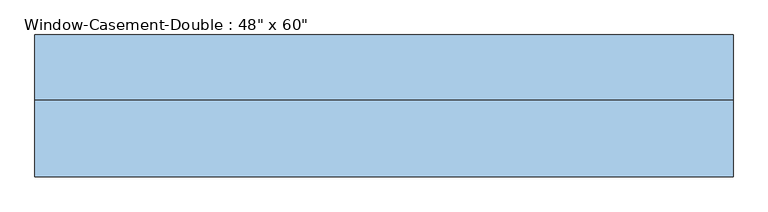
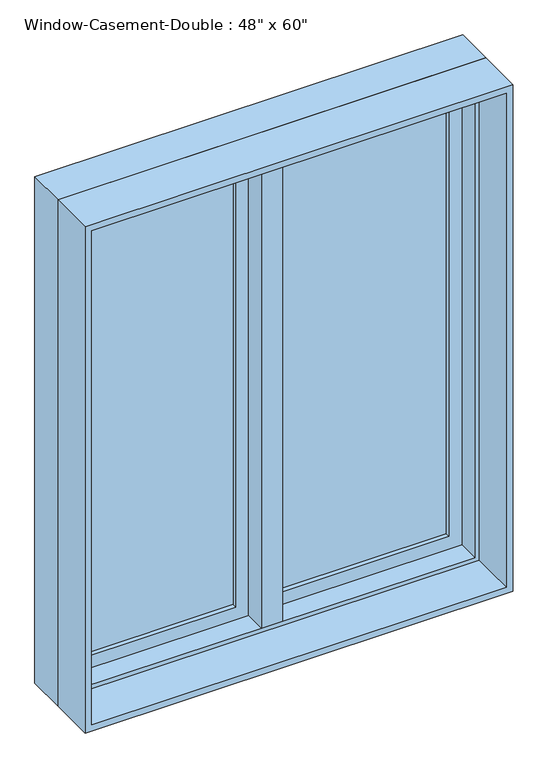
"""IFC4 building model written with IfcOpenShell, lengths in millimetres: window geometry."""

from ifc_helpers import new_model, si_unit, frame, origin, place, context, project, spatial, polyline, outline, extrude, faceted_brep, source, transform, mapped, element, save


def window_8377141f(model_context):
    return source(origin(), model_context, "Body", "SolidModel", [
        faceted_brep([(9.525, 133.35, 2425.7), (-9.525, 133.35, 2425.7), (-9.525, 82.55, 2425.7), (9.525, 82.55, 2425.7), (9.525, 133.35, 927.1), (9.525, 82.55, 927.1), (-9.525, 82.55, 927.1), (-9.525, 133.35, 927.1), (-9.525, 82.55, 946.15), (-9.525, 82.55, 2406.65), (-30.1625, 82.55, 946.15), (-30.1625, 82.55, 2406.65), (-30.1625, 19.05, 946.15), (-30.1625, 19.05, 2406.65), (30.1625, 19.05, 946.15), (30.1625, 19.05, 2406.65), (30.1625, 82.55, 946.15), (30.1625, 82.55, 2406.65), (9.525, 82.55, 946.15), (9.525, 82.55, 2406.65)], [[[0, 1, 2, 3]], [[4, 5, 6, 7]], [[1, 0, 4, 7]], [[2, 1, 7, 6, 8, 9]], [[9, 8, 10, 11]], [[11, 10, 12, 13]], [[13, 12, 14, 15]], [[15, 14, 16, 17]], [[17, 16, 18, 19]], [[0, 3, 19, 18, 5, 4]], [[18, 8, 6, 5]], [[9, 19, 3, 2]], [[8, 18, 16, 14, 12, 10]], [[19, 9, 11, 13, 15, 17]]]),
        extrude(outline(polyline([(-66.675, 114.3), (-66.675, 107.95), (-539.75, 107.95), (-539.75, 114.3), (-66.675, 114.3)])), frame((0.0, 0.0, 984.25), z_axis=(0.0, 0.0, 1.0), x_axis=(1.0, 0.0, 0.0)), (0.0, 0.0, 1.0), 1384.3),
        extrude(outline(polyline([(-539.75, 95.25), (-539.75, 101.6), (-66.675, 101.6), (-66.675, 95.25), (-539.75, 95.25)])), frame((0.0, 0.0, 984.25), z_axis=(0.0, 0.0, 1.0), x_axis=(1.0, 0.0, 0.0)), (0.0, 0.0, 1.0), 1384.3),
        extrude(outline(polyline([(539.75, 114.3), (539.75, 107.95), (66.675, 107.95), (66.675, 114.3), (539.75, 114.3)])), frame((0.0, 0.0, 984.25), z_axis=(0.0, 0.0, 1.0), x_axis=(1.0, 0.0, 0.0)), (0.0, 0.0, 1.0), 1384.3),
        extrude(outline(polyline([(66.675, 95.25), (66.675, 101.6), (539.75, 101.6), (539.75, 95.25), (66.675, 95.25)])), frame((0.0, 0.0, 984.25), z_axis=(0.0, 0.0, 1.0), x_axis=(1.0, 0.0, 0.0)), (0.0, 0.0, 1.0), 1384.3),
        extrude(outline(polyline([(2425.7, -596.9), (927.1, -596.9), (927.1, -9.525), (2425.7, -9.525), (2425.7, -596.9)]), holes=[polyline([(2368.55, -66.675), (984.25, -66.675), (984.25, -539.75), (2368.55, -539.75), (2368.55, -66.675)])]), frame((0.0, 82.55, 0.0), z_axis=(0.0, 1.0, 0.0), x_axis=(0.0, 0.0, 1.0)), (0.0, 0.0, 1.0), 44.45),
        extrude(outline(polyline([(927.1, 596.9), (2425.7, 596.9), (2425.7, 9.525), (927.1, 9.525), (927.1, 596.9)]), holes=[polyline([(984.25, 66.675), (2368.55, 66.675), (2368.55, 539.75), (984.25, 539.75), (984.25, 66.675)])]), frame((0.0, 82.55, 0.0), z_axis=(0.0, 1.0, 0.0), x_axis=(0.0, 0.0, 1.0)), (0.0, 0.0, 1.0), 44.45),
        extrude(outline(polyline([(2438.4, -609.6), (914.4, -609.6), (914.4, 609.6), (2438.4, 609.6), (2438.4, -609.6)]), holes=[polyline([(2419.35, 590.55), (933.45, 590.55), (933.45, -590.55), (2419.35, -590.55), (2419.35, 590.55)])]), frame((0.0, -114.3, 0.0), z_axis=(0.0, 1.0, 0.0), x_axis=(0.0, 0.0, 1.0)), (0.0, 0.0, 1.0), 133.35),
        faceted_brep([(577.85, 82.55, 2406.65), (577.85, 19.05, 2406.65), (-577.85, 19.05, 2406.65), (-577.85, 82.55, 2406.65), (596.9, 133.35, 2425.7), (596.9, 82.55, 2425.7), (-596.9, 82.55, 2425.7), (-596.9, 133.35, 2425.7), (609.6, 19.05, 2438.4), (609.6, 133.35, 2438.4), (-609.6, 133.35, 2438.4), (-609.6, 19.05, 2438.4), (-577.85, 19.05, 946.15), (-577.85, 82.55, 946.15), (-596.9, 82.55, 927.1), (-596.9, 133.35, 927.1), (-609.6, 133.35, 914.4), (-609.6, 19.05, 914.4), (577.85, 19.05, 946.15), (577.85, 82.55, 946.15), (596.9, 82.55, 927.1), (596.9, 133.35, 927.1), (609.6, 133.35, 914.4), (609.6, 19.05, 914.4)], [[[0, 1, 2, 3]], [[4, 5, 6, 7]], [[8, 9, 10, 11]], [[3, 2, 12, 13]], [[7, 6, 14, 15]], [[11, 10, 16, 17]], [[13, 12, 18, 19]], [[15, 14, 20, 21]], [[17, 16, 22, 23]], [[11, 17, 23, 8], [1, 18, 12, 2]], [[19, 18, 1, 0]], [[5, 20, 14, 6], [3, 13, 19, 0]], [[21, 20, 5, 4]], [[23, 22, 9, 8]], [[9, 22, 16, 10], [7, 15, 21, 4]]]),
    ])


if __name__ == "__main__":
    model = new_model("IFC4")
    model_context = context("Model", 3, world=origin())
    ifc_project = project(units=[si_unit("LENGTHUNIT", "METRE", prefix="MILLI")], contexts=[model_context])
    site = spatial("IfcSite", under=ifc_project)
    building = spatial("IfcBuilding", under=site)
    placement = place(None, origin())
    window_shape = window_8377141f(model_context)
    element("IfcWindow", 1, ObjectType="Window-Casement-Double : 48\" x 60\"", at=placement, inside=building, context=model_context, shape_type="MappedRepresentation", body=[
        mapped(window_shape, transform((0.0, 0.0, 0.0), x_axis=(1.0, 0.0, 0.0), y_axis=(0.0, 1.0, 0.0), z_axis=(0.0, 0.0, 1.0))),
    ])
    save(model, "model.ifc")

# Revit data of these elements
# Type "Window-Casement-Double : 48\" x 60\""
#   Type Mark = "17"
#   Fire Rating = "0.5h"
#   Assembly Code = "B2020100"
#   Analytic Construction = "Double glazing - domestic"
#   Frame Extension [instance default] = 0' - 0 1/4"
#   Window Inset [instance default] = 0' - 0"
#   Wall Thickness [instance default] = 0' - 6"
#   Interior Wall Closure [instance default] = 0' - 2 1/4"
#   Half Width = 2' - 0"
#   Visual Light Transmittance = 0.81
#   Thermal Resistance (R) = 1.8146 (h·ft²·°F)/BTU
#   Solar Heat Gain Coefficient = 0.76
#   Rough Width = 4' - 0 1/2"
#   Rough Height = 5' - 0 1/2"
#   Height = 5' - 0"
#   Heat Transfer Coefficient (U) = 0.5511 BTU/(h·ft²·°F)
#   Exterior Wall Closure [instance default] = 0' - 1 1/4"
#   Extension Jamb [instance default] = 0' - 2 1/4"
#   Default Sill Height = 3' - 0"
#   Width = 4' - 0"
#   Define Thermal Properties by = 0
#   Muntin Visibility = yes
#   Interior Trim Visibility [instance default] = yes
#   Exterior Trim Visibility [instance default] = yes
#   Extension Jamb Visibility [instance default] = yes
#   Interior Trim Material = Wood - Stained
#   Muntin Pattern = Muntin Pattern_2x2 : Muntin Pattern_2x2
#   Interior Trim = Trim-Window-Interior-Flat : Picture Frame
#   Interior Frame Material = Wood - Stained
#   Glass Panel Material = Glass
#   Exterior Trim Material = Clad - White
#   Exterior Trim = Trim-Window-Exterior-Flat : with Sill
#   Exterior Frame Material = Clad - White
#   Wall Closure = (empty or 0)
# Element 1 (IfcWindow, "Window-Casement-Double : 48\" x 60\"")
#   Wall Thickness = 0' - 9"
#   Extension Jamb = 0' - 5 1/4"
#   Materials on its faces: "Wood - Stained", "Glass", "Clad - White"
# Materials
#   "Wood - Stained": class "Wood", colour RGB 224 178 126, transparency 0, Cost = 0
#   "Glass": class "Glass", colour RGB 0 128 192, transparency 0.75, Description = "Soda Lime Glass", Cost = 0
#   "Clad - White": class "Wood", colour RGB 242 242 238, transparency 0, Cost = 0
